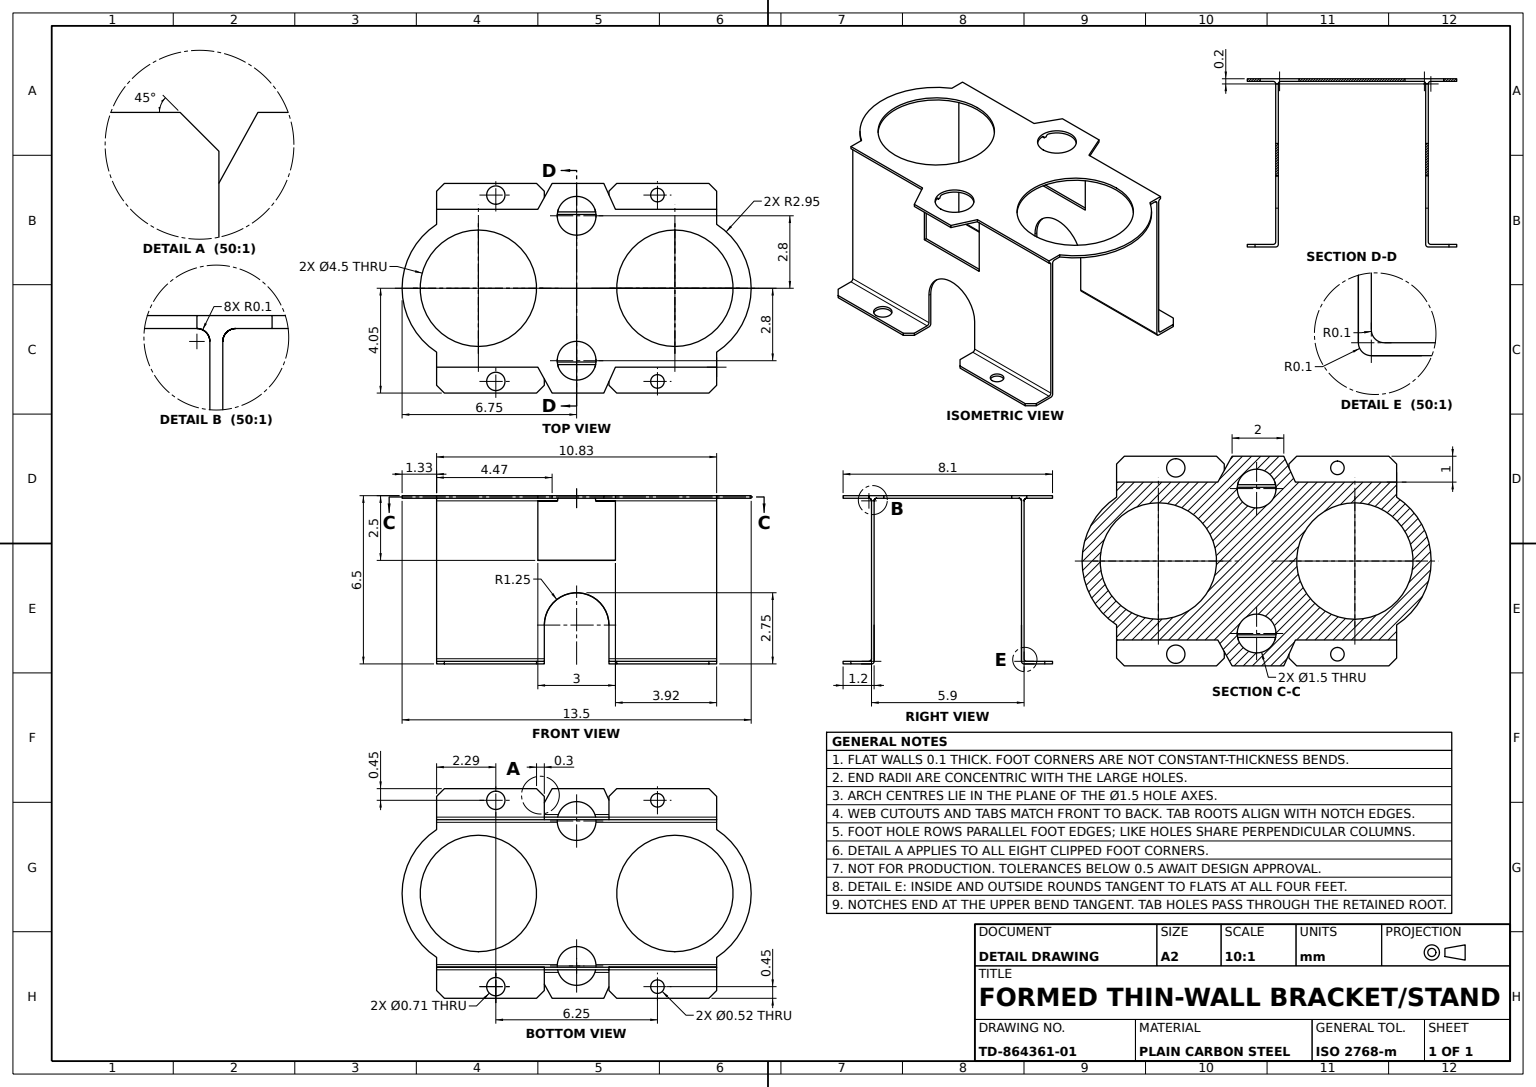
from build123d import *

# Parameters (mm, degrees)
BRACKET_CHANNEL_BODY_DEPTH     = 5.415
SIDE_ARCH_CUT_A_DEPTH          = 10.83
SIDE_WINDOW_CUT_SKETCH_W       = 2.5
SIDE_WINDOW_CUT_SKETCH_H       = 0.2
SIDE_WINDOW_CUT_DEPTH          = 10.83
SIDE_ARCH_CUT_B_SKETCH_W       = 3
SIDE_ARCH_CUT_B_SKETCH_H       = 2.3
SIDE_ARCH_CUT_B_DEPTH          = 10.83
TOP_PLATE_LUGS_DEPTH           = 0.1
LUG_TRIM_CUT_SKETCH_R          = 2.25
LUG_TRIM_CUT_DEPTH             = 0.1
LARGE_HOLES_2XD2_8_SKETCH_R    = 0.75
LARGE_HOLES_2XD2_8_DEPTH       = 0.1
HOLE_CUT_A_SKETCH_R            = 0.75
HOLE_CUT_A_DEPTH               = 0.1
PROFILE_TRIM_CUT_DEPTH         = 0.1
SMALL_HOLES_2XD0_45_SKETCH_R   = 0.261538798
SMALL_HOLES_2XD0_45_SKETCH_R_2 = 0.354559983
SMALL_HOLES_2XD0_45_DEPTH      = 0.1
HOLE_CUT_B_SKETCH_R            = 0.75
HOLE_CUT_B_DEPTH               = 0.1
EDGE_CHAMFER_0_3_SIZE          = 0.3
ARCH_EDGE_CHAMFER_0_3_SIZE     = 0.3


with BuildPart() as part:
    # Channel Profile Sketch → Bracket Channel Body (new, symmetric)
    with BuildSketch(Plane.XY):
        with BuildLine():
            ThreePointArc((-2.95, 0), (-2.879289322, 0.029289322), (-2.85, 0.1))
            Line((-2.85, 0.1), (-2.85, 6.3))
            ThreePointArc((-2.85, 6.3), (-2.820710678, 6.370710678), (-2.75, 6.4))
            Line((-2.75, 6.4), (2.75, 6.4))
            ThreePointArc((2.75, 6.4), (2.820710678, 6.370710678), (2.85, 6.3))
            Line((2.85, 6.3), (2.85, 0.1))
            ThreePointArc((2.85, 0.1), (2.879289322, 0.029289322), (2.95, 0))
            Line((2.95, 0), (4.05, 0))
            Line((4.05, 0), (4.05, 0.1))
            Line((4.05, 0.1), (3.05, 0.1))
            ThreePointArc((3.05, 0.1), (2.979289322, 0.129289322), (2.95, 0.2))
            Line((2.95, 0.2), (2.95, 6.3))
            ThreePointArc((2.95, 6.3), (2.979289322, 6.370710678), (3.05, 6.4))
            Line((3.05, 6.4), (4.05, 6.4))
            Line((4.05, 6.4), (4.05, 6.5))
            Line((4.05, 6.5), (-4.05, 6.5))
            Line((-4.05, 6.5), (-4.05, 6.4))
            Line((-4.05, 6.4), (-3.05, 6.4))
            ThreePointArc((-3.05, 6.4), (-2.979289322, 6.370710678), (-2.95, 6.3))
            Line((-2.95, 6.3), (-2.95, 0.2))
            ThreePointArc((-2.95, 0.2), (-2.979289322, 0.129289322), (-3.05, 0.1))
            Line((-3.05, 0.1), (-4.05, 0.1))
            Line((-4.05, 0.1), (-4.05, 0))
            Line((-4.05, 0), (-2.95, 0))
        make_face()
    extrude(amount=BRACKET_CHANNEL_BODY_DEPTH, both=True)

    # Side Arch Cut A Sketch → Side Arch Cut A (cut)
    with BuildSketch(Plane(origin=(2.95, 0, 0), x_dir=(0, 0, -1), z_dir=(1, 0, 0))):
        with BuildLine():
            Line((-1.25, 1.5), (-1.25, 0))
            Line((-1.25, 0), (1.25, 0))
            Line((1.25, 0), (1.25, 1.5))
            ThreePointArc((1.25, 1.5), (0, 2.75), (-1.25, 1.5))
        make_face()
    extrude(amount=-SIDE_ARCH_CUT_A_DEPTH, mode=Mode.SUBTRACT)

    # Side Window Cut Sketch → Side Window Cut (cut)
    with BuildSketch(Plane.ZY.offset(2.95)):
        with Locations((0, 0.1)):
            Rectangle(SIDE_WINDOW_CUT_SKETCH_W, SIDE_WINDOW_CUT_SKETCH_H)
    extrude(amount=-SIDE_WINDOW_CUT_DEPTH, mode=Mode.SUBTRACT)

    # Side Arch Cut B Sketch → Side Arch Cut B (cut)
    with BuildSketch(Plane(origin=(2.95, 0, 0), x_dir=(0, 0, -1), z_dir=(1, 0, 0))):
        with Locations((0, 5.15)):
            Rectangle(SIDE_ARCH_CUT_B_SKETCH_W, SIDE_ARCH_CUT_B_SKETCH_H)
    extrude(amount=-SIDE_ARCH_CUT_B_DEPTH, mode=Mode.SUBTRACT)

    # Top Plate Lugs Sketch → Top Plate Lugs (add)
    with BuildSketch(Plane(origin=(0, 6.5, 0), x_dir=(1, 0, 0), z_dir=(0, 1, 0))):
        with BuildLine():
            Line((-2.468658543, 5.415), (-1.566612588, 5.415))
            ThreePointArc((-1.566612588, 5.415), (0, 6.05), (1.566612588, 5.415))
            Line((1.566612588, 5.415), (2.468658543, 5.415))
            ThreePointArc((2.468658543, 5.415), (0, 6.75), (-2.468658543, 5.415))
        make_face()
        with BuildLine():
            Line((-2.468658543, -5.415), (-1.566612588, -5.415))
            ThreePointArc((-1.566612588, -5.415), (0, -6.05), (1.566612588, -5.415))
            Line((1.566612588, -5.415), (2.468658543, -5.415))
            ThreePointArc((2.468658543, -5.415), (0, -6.75), (-2.468658543, -5.415))
        make_face()
    extrude(amount=-TOP_PLATE_LUGS_DEPTH)

    # Lug Trim Cut Sketch → Lug Trim Cut (cut)
    with BuildSketch(Plane(origin=(0, 6.5, 0), x_dir=(1, 0, 0), z_dir=(0, 1, 0))):
        with Locations(Location((0, 3.8, 0), (0, 0, 180))):
            Circle(LUG_TRIM_CUT_SKETCH_R)
        with Locations(Location((0, -3.8, 0), (0, 0, 180))):
            Circle(LUG_TRIM_CUT_SKETCH_R)
    extrude(amount=-LUG_TRIM_CUT_DEPTH, mode=Mode.SUBTRACT)

    # Large Holes 2xD2.8 Sketch → Large Holes 2xD2.8 (cut)
    with BuildSketch(Plane(origin=(0, 6.5, 0), x_dir=(1, 0, 0), z_dir=(0, 1, 0))):
        with Locations(Location((2.8, 0, 0), (0, 0, 180))):
            Circle(LARGE_HOLES_2XD2_8_SKETCH_R)
        with Locations(Location((-2.8, 0, 0), (0, 0, 180))):
            Circle(LARGE_HOLES_2XD2_8_SKETCH_R)
    extrude(amount=-LARGE_HOLES_2XD2_8_DEPTH, mode=Mode.SUBTRACT)

    # Hole Cut A Sketch → Hole Cut A (cut)
    with BuildSketch(Plane(origin=(0, 6.4, 0), x_dir=(1, 0, 0), z_dir=(0, 1, 0))):
        with Locations(Location((2.8, 0, 0), (0, 0, 180))):
            Circle(HOLE_CUT_A_SKETCH_R)
    extrude(amount=-HOLE_CUT_A_DEPTH, mode=Mode.SUBTRACT)

    # Profile Trim Cut Sketch → Profile Trim Cut (cut)
    with BuildSketch(Plane(origin=(0, 6.5, 0), x_dir=(1, 0, 0), z_dir=(0, 1, 0))):
        Polygon((-4.05, 1.051616968), (-3.05, 1.5), (-3.05, 5.415), (-4.05, 5.415), align=None)
        Polygon((-4.05, -0.948383032), (-3.05, -1.5), (-3.05, -5.415), (-4.05, -5.415), align=None)
        Polygon((3.05, -1.5), (3.05, -5.415), (4.05, -5.415), (4.05, -0.948383032), align=None)
        Polygon((4.05, 5.415), (4.05, 1.051616968), (3.05, 1.5), (3.05, 5.415), align=None)
    extrude(amount=-PROFILE_TRIM_CUT_DEPTH, mode=Mode.SUBTRACT)

    # Small Holes 2xD0.45 Sketch → Small Holes 2xD0.45 (cut)
    with BuildSketch(Plane(origin=(0, 0.1, 0), x_dir=(1, 0, 0), z_dir=(0, 1, 0))):
        with Locations(Location((3.6, 3.125, 0), (0, 0, 180))):
            Circle(SMALL_HOLES_2XD0_45_SKETCH_R)
        with Locations(Location((3.6, -3.125, 0), (0, 0, 180))):
            Circle(SMALL_HOLES_2XD0_45_SKETCH_R_2)
        with Locations((-3.6, -3.125)):
            Circle(SMALL_HOLES_2XD0_45_SKETCH_R_2)
        with Locations((-3.6, 3.125)):
            Circle(SMALL_HOLES_2XD0_45_SKETCH_R)
    extrude(amount=-SMALL_HOLES_2XD0_45_DEPTH, mode=Mode.SUBTRACT)

    # Hole Cut B Sketch → Hole Cut B (cut)
    with BuildSketch(Plane(origin=(0, 6.4, 0), x_dir=(1, 0, 0), z_dir=(0, 1, 0))):
        with Locations(Location((-2.8, 0, 0), (0, 0, 180))):
            Circle(HOLE_CUT_B_SKETCH_R)
    extrude(amount=-HOLE_CUT_B_DEPTH, mode=Mode.SUBTRACT)

    # Edge Chamfer 0.3
    edge_chamfer_0_3_edges = [part.edges().sort_by_distance(p)[0] for p in [
        (4.05, 0.05, 5.415),
    ]]
    chamfer(edge_chamfer_0_3_edges, length=EDGE_CHAMFER_0_3_SIZE)

    # Arch Edge Chamfer 0.3
    arch_edge_chamfer_0_3_edges = [part.edges().sort_by_distance(p)[0] for p in [
        (4.05, 0.05, 1.25),
        (4.05, 0.05, -1.25),
        (-4.05, 0.05, -5.415),
        (4.05, 0.05, -5.415),
        (-4.05, 0.05, 5.415),
        (-4.05, 0.05, -1.25),
        (-4.05, 0.05, 1.25),
    ]]
    chamfer(arch_edge_chamfer_0_3_edges, length=ARCH_EDGE_CHAMFER_0_3_SIZE)


solid = part.part
